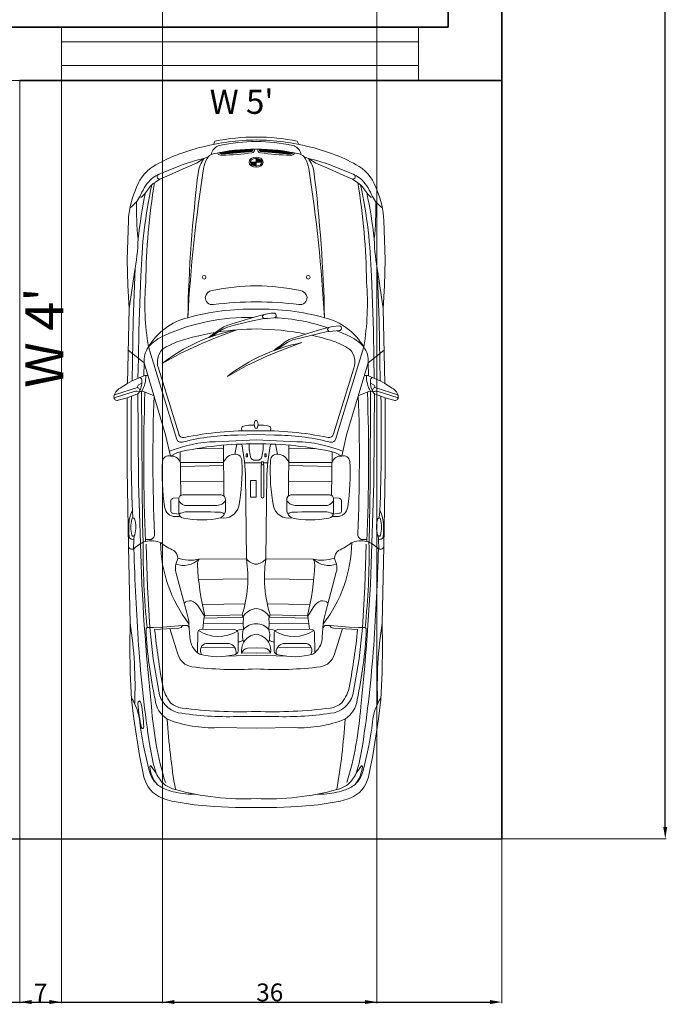
# Model space of a CAD drawing. Units: feet. Extents: x -297 to 770, y -228 to 625.
# Tile 4 of 14: x 661 to 770, y -228 to -62. Entities that reach past the tile are written whole.
import ezdxf

# ---------------------------------------------------------------- set-up
doc = ezdxf.new("R2010")
doc.units = ezdxf.units.FT
doc.header["$MEASUREMENT"] = 0
for name, color, linetype, lineweight in [('A-ANNO-DIMS', 2, 'Continuous', 18), ('A-ANNO-TEXT', 7, 'Continuous', 18), ('A-EQPM-VEHI', 8, 'Continuous', 13), ('A-EQPM-VEHI-PATT', 9, 'Continuous', 13), ('A-FLOR-EDGE', 7, 'Continuous', 25), ('A-WALL', 7, 'Continuous', 35), ('windows', 30, 'Continuous', 18)]:
    doc.layers.add(name, color=color, linetype=linetype, lineweight=lineweight)
doc.styles.add('Annotative', font='arial.ttf')
doc.styles.get("Standard").update_dxf_attribs({"font": 'arial.ttf'})
doc.dimstyles.get("Standard").update_dxf_attribs({"dimtxt": 3, "dimasz": 2, "dimexe": 0.18, "dimexo": 0.0625, "dimgap": 0.09, "dimtad": 1, "dimtoh": 1, "dimdec": 1, "dimzin": 0, "dimdsep": 46, "dimlunit": 3, "dimtxsty": 'Standard', "dimcen": 0, "dimclre": 256, "dimadec": 0, "dimazin": 0, "dimtfac": 1, "dimtdec": 1, "dimtofl": 0, "dimtmove": 0, "dimatfit": 3, "dimfxl": 1, "dimtolj": 1, "dimtzin": 0, "dimlwe": -1, "dimarcsym": 0})

# ---------------------------------------------------------------- blocks, each defined once
blk = doc.blocks.new('WIN-5FT')
for p, q in [((60, 6.5), (0, 6.5)), ((60, 2.5), (0, 2.5))]:
    blk.add_line(p, q)
blk.add_lwpolyline([(60, 0), (60, 9), (0, 9), (0, 0)], close=True)
blk = doc.blocks.new('*D43')
at = {"layer": 'A-ANNO-DIMS', "transparency": 16777216}
for p, q in [((382.16, -173.1), (382.16, -227.67)), ((742.16, -200.1), (742.16, -227.67))]:
    blk.add_line(p, q, dxfattribs=at)
at = {"layer": 'A-ANNO-DIMS', "color": 0, "lineweight": -2, "transparency": 16777216}
blk.add_line((384.16, -227.49), (740.16, -227.49), dxfattribs=at)
at = {"layer": 'A-ANNO-DIMS', "color": 0, "transparency": 16777216}
for points in [[(384.16, -227.15), (384.16, -227.82), (382.16, -227.49)], [(740.16, -227.15), (740.16, -227.82), (742.16, -227.49)]]:
    blk.add_solid(points, dxfattribs=at)
at = {"layer": 'Defpoints', "color": 0, "transparency": 16777216}
for p in [(382.16, -173.04), (742.16, -200.04), (742.16, -227.49)]:
    blk.add_point(p, dxfattribs=at)
at = {"layer": 'A-ANNO-DIMS', "color": 0, "transparency": 16777216, "insert": (562.16, -225.86), "char_height": 3, "attachment_point": 5}
blk.add_mtext('\\A1;360', dxfattribs=at)
blk = doc.blocks.new('*D44')
at = {"layer": 'A-ANNO-DIMS', "transparency": 16777216}
for p, q in [((742.22, 306.96), (769.79, 306.96)), ((742.22, -200.04), (769.79, -200.04))]:
    blk.add_line(p, q, dxfattribs=at)
at = {"layer": 'A-ANNO-DIMS', "color": 0, "lineweight": -2, "transparency": 16777216}
blk.add_line((769.61, -198.04), (769.61, 304.96), dxfattribs=at)
at = {"layer": 'A-ANNO-DIMS', "color": 0, "transparency": 16777216}
for points in [[(769.27, 304.96), (769.94, 304.96), (769.61, 306.96)], [(769.27, -198.04), (769.94, -198.04), (769.61, -200.04)]]:
    blk.add_solid(points, dxfattribs=at)
at = {"layer": 'Defpoints', "color": 0, "transparency": 16777216}
for p in [(742.16, 306.96), (769.61, 306.96), (742.16, -200.04)]:
    blk.add_point(p, dxfattribs=at)
at = {"layer": 'A-ANNO-DIMS', "color": 0, "transparency": 16777216, "insert": (767.98, 53.46), "char_height": 3, "attachment_point": 5, "rotation": 90}
blk.add_mtext('\\A1;507', dxfattribs=at)
blk = doc.blocks.new('*D56')
at = {"layer": 'A-ANNO-DIMS', "transparency": 16777216}
for p, q in [((742.09, -72.54), (354.53, -72.54)), ((742.09, -200.04), (354.53, -200.04))]:
    blk.add_line(p, q, dxfattribs=at)
at = {"layer": 'A-ANNO-DIMS', "color": 0, "lineweight": -2, "transparency": 16777216}
blk.add_line((354.71, -74.54), (354.71, -198.04), dxfattribs=at)
at = {"layer": 'A-ANNO-DIMS', "color": 0, "transparency": 16777216}
for points in [[(354.37, -74.54), (355.04, -74.54), (354.71, -72.54)], [(354.37, -198.04), (355.04, -198.04), (354.71, -200.04)]]:
    blk.add_solid(points, dxfattribs=at)
at = {"layer": 'Defpoints', "color": 0, "transparency": 16777216}
for p in [(742.16, -72.54), (354.71, -200.04), (742.16, -200.04)]:
    blk.add_point(p, dxfattribs=at)
at = {"layer": 'A-ANNO-DIMS', "color": 0, "transparency": 16777216, "insert": (353.08, -136.29), "char_height": 3, "attachment_point": 5, "rotation": 90}
blk.add_mtext('\\A1;127.5', dxfattribs=at)
blk = doc.blocks.new('*D58')
at = {"layer": 'A-ANNO-DIMS', "transparency": 16777216}
for p, q in [((661.16, -72.6), (661.16, -227.67)), ((668.16, -72.6), (668.16, -227.67))]:
    blk.add_line(p, q, dxfattribs=at)
at = {"layer": 'A-ANNO-DIMS', "color": 0, "lineweight": -2, "transparency": 16777216}
blk.add_line((663.16, -227.49), (666.16, -227.49), dxfattribs=at)
at = {"layer": 'A-ANNO-DIMS', "color": 0, "transparency": 16777216}
for points in [[(663.16, -227.15), (663.16, -227.82), (661.16, -227.49)], [(666.16, -227.15), (666.16, -227.82), (668.16, -227.49)]]:
    blk.add_solid(points, dxfattribs=at)
at = {"layer": 'Defpoints', "color": 0, "transparency": 16777216}
for p in [(661.16, -72.54), (668.16, -72.54), (668.16, -227.49)]:
    blk.add_point(p, dxfattribs=at)
at = {"layer": 'A-ANNO-DIMS', "color": 0, "transparency": 16777216, "insert": (664.66, -225.9), "char_height": 3, "attachment_point": 5}
blk.add_mtext('\\A1;7', dxfattribs=at)
blk = doc.blocks.new('*D68')
at = {"layer": 'A-ANNO-DIMS', "transparency": 16777216}
for p, q in [((685.16, 306.9), (685.16, -227.67)), ((721.16, 306.9), (721.16, -227.67))]:
    blk.add_line(p, q, dxfattribs=at)
at = {"layer": 'A-ANNO-DIMS', "color": 0, "lineweight": -2, "transparency": 16777216}
blk.add_line((687.16, -227.49), (719.16, -227.49), dxfattribs=at)
at = {"layer": 'A-ANNO-DIMS', "color": 0, "transparency": 16777216}
for points in [[(687.16, -227.15), (687.16, -227.82), (685.16, -227.49)], [(719.16, -227.15), (719.16, -227.82), (721.16, -227.49)]]:
    blk.add_solid(points, dxfattribs=at)
at = {"layer": 'Defpoints', "color": 0, "transparency": 16777216}
for p in [(685.16, 306.96), (721.16, 306.96), (721.16, -227.49)]:
    blk.add_point(p, dxfattribs=at)
at = {"layer": 'A-ANNO-DIMS', "color": 0, "transparency": 16777216, "insert": (703.16, -225.86), "char_height": 3, "attachment_point": 5}
blk.add_mtext('\\A1;36', dxfattribs=at)

msp = doc.modelspace()

# ---------------------------------------------------------------- hatches: boundary and pattern name
at = {"layer": 'A-EQPM-VEHI-PATT'}
h = msp.add_hatch(dxfattribs=at)
h.set_pattern_fill('ANSI31', color=256, scale=0.200946, angle=30.004, style=0)
h.set_pattern_definition([(75.004, (382.155307, -173.037275), (-0.0242628202, 0.0064993876), [])])
h.paths.add_polyline_path([(694.646, -84.653), (694.683, -84.701), (694.726, -84.744), (694.774, -84.781), (694.826, -84.813), (694.881, -84.837), (694.939, -84.854), (694.999, -84.864), (695.059, -84.866), (695.12, -84.861), (695.681, -84.839), (696.241, -84.812), (696.801, -84.778), (697.361, -84.738), (697.921, -84.691), (698.479, -84.639), (699.038, -84.58), (699.595, -84.514), (700.152, -84.443), (700.189, -84.437), (700.225, -84.425), (700.258, -84.407), (700.287, -84.382), (700.31, -84.353), (700.329, -84.32), (700.34, -84.284), (700.345, -84.247), (700.343, -84.209), (700.334, -84.173), (700.319, -84.139), (700.297, -84.108), (700.27, -84.081), (700.239, -84.06), (700.126, -84.063), (700.014, -84.066), (699.901, -84.069), (699.789, -84.073), (699.676, -84.077), (699.564, -84.082), (699.451, -84.086), (699.339, -84.092), (699.226, -84.097), (699.114, -84.103), (699.001, -84.11), (698.889, -84.116), (698.776, -84.124), (698.664, -84.131), (698.552, -84.139), (698.439, -84.147), (698.327, -84.156), (698.215, -84.165), (698.103, -84.174), (697.991, -84.184), (697.878, -84.194), (697.766, -84.205), (697.654, -84.216), (697.542, -84.227), (697.43, -84.239), (697.318, -84.251), (697.206, -84.263), (697.094, -84.276), (696.983, -84.289), (696.871, -84.303), (696.759, -84.317), (696.647, -84.331), (696.536, -84.346), (696.424, -84.361), (696.313, -84.376), (696.201, -84.392), (696.09, -84.408), (695.978, -84.425), (695.867, -84.442), (695.756, -84.459), (695.644, -84.477), (695.533, -84.495), (695.422, -84.513), (695.311, -84.532), (695.2, -84.551), (695.089, -84.571), (694.979, -84.591), (694.868, -84.611), (694.757, -84.632)])
h = msp.add_hatch(dxfattribs=at)
h.set_pattern_fill('ANSI31', color=256, scale=0.200942, angle=30.004, style=0)
h.set_pattern_definition([(75.004, (382.155307, -173.037275), (-0.0242623372, 0.0064992583), [])])
h.paths.add_polyline_path([(701.519, -84.06), (701.488, -84.081), (701.461, -84.108), (701.439, -84.139), (701.424, -84.173), (701.415, -84.209), (701.413, -84.247), (701.418, -84.284), (701.429, -84.32), (701.448, -84.353), (701.471, -84.382), (701.5, -84.407), (701.533, -84.425), (701.569, -84.437), (701.606, -84.443), (702.163, -84.514), (702.72, -84.58), (703.278, -84.639), (703.837, -84.691), (704.397, -84.738), (704.956, -84.778), (705.517, -84.812), (706.077, -84.839), (706.638, -84.861), (706.699, -84.866), (706.759, -84.864), (706.819, -84.854), (706.877, -84.837), (706.932, -84.813), (706.984, -84.781), (707.032, -84.744), (707.075, -84.701), (707.111, -84.653), (707.001, -84.632), (706.89, -84.611), (706.779, -84.591), (706.669, -84.571), (706.558, -84.551), (706.447, -84.532), (706.336, -84.513), (706.225, -84.495), (706.113, -84.477), (706.002, -84.459), (705.891, -84.442), (705.78, -84.425), (705.668, -84.408), (705.557, -84.392), (705.445, -84.376), (705.334, -84.361), (705.222, -84.346), (705.111, -84.331), (704.999, -84.317), (704.887, -84.303), (704.775, -84.289), (704.664, -84.276), (704.552, -84.263), (704.44, -84.251), (704.328, -84.239), (704.216, -84.227), (704.104, -84.216), (703.992, -84.205), (703.88, -84.194), (703.767, -84.184), (703.655, -84.174), (703.543, -84.165), (703.431, -84.156), (703.318, -84.147), (703.206, -84.139), (703.094, -84.131), (702.981, -84.124), (702.869, -84.116), (702.757, -84.11), (702.644, -84.103), (702.532, -84.097), (702.419, -84.092), (702.307, -84.086), (702.194, -84.082), (702.082, -84.077), (701.969, -84.073), (701.857, -84.069), (701.744, -84.066), (701.632, -84.063)])
h = msp.add_hatch(color=256, dxfattribs=at)
edge = h.paths.add_edge_path()
edge.add_line((700.879, -86.271), (700.879, -85.631))
edge.add_spline(control_points=[(700.879, -85.631), (701.04, -85.631), (701.2, -85.658), (701.678, -85.83), (701.857, -86.049), (701.857, -86.271)], knot_values=[6.2672483, 6.2672483, 6.2672483, 6.2672483, 6.732595, 6.732595, 7.8539816, 7.8539816, 7.8539816, 7.8539816], degree=3, periodic=0)
edge.add_line((701.857, -86.271), (700.879, -86.271))
h = msp.add_hatch(color=256, dxfattribs=at)
edge = h.paths.add_edge_path()
edge.add_line((700.879, -86.271), (700.879, -86.915))
edge.add_spline(control_points=[(700.879, -86.915), (700.553, -86.915), (700.236, -86.793), (699.955, -86.516), (699.902, -86.393), (699.901, -86.271)], knot_values=[4.712389, 4.712389, 4.712389, 4.712389, 5.655061, 5.655061, 6.2672483, 6.2672483, 6.2672483, 6.2672483], degree=3, periodic=0)
edge.add_line((699.901, -86.271), (700.879, -86.271))

# ---------------------------------------------------------------- linework, layer by layer
at = {"layer": 'A-EQPM-VEHI'}
for p, q in [((693.964, -82.748), (693.722, -83.283)), ((707.794, -82.748), (708.036, -83.283)), ((688.627, -86.65), (690.666, -85.978)), ((690.666, -85.978), (692.112, -85.668)), ((692.112, -85.668), (690.847, -86.443)), ((692.112, -85.668), (692.817, -85.365)), ((693.4, -84.666), (693.386, -84.944)), ((700.879, -85.631), (700.879, -86.915)), ((708.358, -84.666), (708.372, -84.944)), ((709.646, -85.668), (708.941, -85.365)), ((711.091, -85.978), (709.646, -85.668)), ((709.646, -85.668), (710.911, -86.443)), ((713.131, -86.65), (711.091, -85.978)), ((685.115, -88.07), (688.627, -86.65)), ((688.601, -87.399), (686.251, -88.432)), ((690.847, -86.443), (688.601, -87.399)), ((699.901, -86.271), (700.879, -86.271)), ((701.857, -86.271), (700.879, -86.271)), ((710.911, -86.443), (713.157, -87.399)), ((716.642, -88.07), (713.131, -86.65)), ((713.157, -87.399), (715.506, -88.432)), ((684.702, -89.129), (683.954, -89.646)), ((686.251, -88.432), (684.702, -89.129)), ((715.506, -88.432), (717.056, -89.129)), ((717.056, -89.129), (717.804, -89.646)), ((682.766, -90.73), (682.095, -91.634)), ((718.992, -90.73), (719.663, -91.634)), ((682.095, -91.634), (681.682, -92.074)), ((719.663, -91.634), (720.076, -92.074)), ((679.41, -96.044), (679.227, -102.695)), ((722.348, -96.044), (722.531, -102.695)), ((679.227, -102.695), (679.313, -106.998)), ((680.554, -104.049), (680.201, -112.961)), ((721.204, -104.049), (721.557, -112.961)), ((722.531, -102.695), (722.445, -106.998)), ((680.416, -104.781), (679.518, -110.872)), ((681.527, -105.38), (681.191, -114.601)), ((720.231, -105.38), (720.567, -114.601)), ((721.341, -104.781), (722.24, -110.872)), ((679.313, -106.998), (679.518, -110.872)), ((722.445, -106.998), (722.24, -110.872)), ((679.518, -110.872), (679.278, -123.501)), ((722.24, -110.872), (722.48, -123.501)), ((701.337, -112.092), (699.617, -112.581)), ((702.518, -111.823), (701.337, -112.092)), ((701.69, -112.654), (702.142, -112.562)), ((701.926, -112.216), (701.94, -112.101)), ((701.998, -112.408), (701.926, -112.216)), ((701.94, -112.101), (702.051, -111.963)), ((702.142, -112.562), (701.998, -112.408)), ((702.051, -111.963), (702.166, -111.903)), ((702.142, -112.562), (702.791, -112.543)), ((703.381, -111.678), (702.518, -111.823)), ((702.791, -112.543), (703.835, -112.436)), ((703.796, -111.654), (703.381, -111.678)), ((703.796, -111.654), (703.796, -111.654)), ((703.835, -112.436), (703.835, -112.436)), ((680.201, -112.961), (680.046, -123.059)), ((695.455, -113.938), (694.814, -114.343)), ((695.265, -114.368), (696.073, -113.996)), ((695.973, -113.737), (695.455, -113.938)), ((699.617, -112.581), (695.973, -113.737)), ((696.073, -113.996), (697.228, -113.689)), ((697.228, -113.689), (700.282, -112.955)), ((700.282, -112.955), (701.69, -112.654)), ((713.481, -113.979), (712.3, -114.248)), ((712.903, -114.257), (713.014, -114.119)), ((713.014, -114.119), (713.129, -114.059)), ((714.344, -113.834), (713.481, -113.979)), ((714.759, -113.81), (714.344, -113.834)), ((714.759, -113.81), (714.759, -113.81)), ((721.557, -112.961), (721.712, -123.059)), ((681.191, -114.601), (681.09, -119.232)), ((691.732, -116.744), (694.354, -115.672)), ((693.249, -115.488), (692.949, -115.758)), ((694.092, -114.854), (693.249, -115.488)), ((693.411, -115.59), (694.295, -114.964)), ((694.814, -114.343), (694.092, -114.854)), ((694.295, -114.964), (695.265, -114.368)), ((694.354, -115.672), (697.617, -114.453)), ((710.58, -114.736), (706.936, -115.893)), ((707.036, -116.152), (708.191, -115.845)), ((708.191, -115.845), (711.245, -115.11)), ((712.3, -114.248), (710.58, -114.736)), ((711.245, -115.11), (712.653, -114.81)), ((712.653, -114.81), (713.105, -114.718)), ((712.889, -114.372), (712.903, -114.257)), ((712.961, -114.564), (712.889, -114.372)), ((713.105, -114.718), (712.961, -114.564)), ((713.105, -114.718), (713.754, -114.699)), ((713.754, -114.699), (714.798, -114.592)), ((714.798, -114.592), (714.798, -114.592)), ((720.567, -114.601), (720.668, -119.232)), ((682.792, -117.339), (687.544, -132.898)), ((688.215, -118.368), (691.732, -116.744)), ((705.055, -117.01), (704.212, -117.644)), ((704.374, -117.746), (705.258, -117.12)), ((705.777, -116.499), (705.055, -117.01)), ((705.258, -117.12), (706.228, -116.524)), ((705.317, -117.828), (708.58, -116.609)), ((706.418, -116.093), (705.777, -116.499)), ((706.228, -116.524), (707.036, -116.152)), ((706.936, -115.893), (706.418, -116.093)), ((718.966, -117.339), (714.214, -132.898)), ((679.385, -117.896), (682.085, -120.012)), ((685.087, -120.129), (688.215, -118.368)), ((699.178, -120.524), (702.695, -118.9)), ((702.695, -118.9), (705.317, -117.828)), ((704.212, -117.644), (703.912, -117.914)), ((722.373, -117.896), (719.673, -120.012)), ((681.09, -119.232), (681.028, -122.633)), ((682.085, -120.012), (682.008, -122.207)), ((682.085, -120.012), (685.674, -132.099)), ((696.05, -122.285), (699.178, -120.524)), ((719.673, -120.012), (716.084, -132.099)), ((719.673, -120.012), (719.75, -122.207)), ((720.668, -119.232), (720.73, -122.633)), ((682.008, -122.207), (680.046, -123.059)), ((684.446, -120.889), (687.88, -131.917)), ((717.312, -120.889), (713.878, -131.917)), ((719.75, -122.207), (721.712, -123.059)), ((680.921, -124.168), (677.075, -125.393)), ((679.278, -123.501), (678.008, -124.278)), ((680.046, -123.059), (679.278, -123.501)), ((681.675, -123.437), (681.069, -123.783)), ((720.083, -123.437), (720.689, -123.783)), ((720.837, -124.168), (724.683, -125.393)), ((721.712, -123.059), (722.48, -123.501)), ((722.48, -123.501), (723.75, -124.278)), ((680.363, -124.8), (677.008, -125.91)), ((680.827, -125.275), (679.191, -125.879)), ((681.015, -125.181), (681.055, -131.504)), ((681.643, -124.752), (681.703, -140.477)), ((683.722, -125.526), (681.958, -124.821)), ((718.036, -125.526), (719.8, -124.821)), ((720.115, -124.752), (720.055, -140.477)), ((720.743, -125.181), (720.703, -131.504)), ((720.931, -125.275), (722.567, -125.879)), ((721.395, -124.8), (724.75, -125.91)), ((679.191, -125.879), (677.724, -126.293)), ((679.191, -125.879), (679.208, -137.861)), ((722.567, -125.879), (722.55, -137.861)), ((722.567, -125.879), (724.034, -126.293)), ((700.722, -129.728), (700.985, -129.728)), ((681.055, -131.504), (681.136, -140.234)), ((685.674, -132.099), (686.5, -135.689)), ((697.788, -132.186), (700.879, -132.078)), ((698.44, -131.022), (698.447, -131.436)), ((700.714, -130.985), (701.022, -130.985)), ((703.97, -132.186), (700.879, -132.078)), ((703.318, -131.022), (703.311, -131.436)), ((716.084, -132.099), (715.258, -135.689)), ((720.703, -131.504), (720.622, -140.234)), ((694.063, -133.266), (700.879, -132.969)), ((695.399, -133.836), (695.427, -142.379)), ((697.651, -133.684), (697.275, -135.367)), ((698.935, -136.618), (698.468, -133.651)), ((707.695, -133.266), (700.879, -132.969)), ((702.823, -136.618), (703.29, -133.651)), ((704.107, -133.684), (704.483, -135.367)), ((706.359, -133.836), (706.331, -142.379)), ((687.681, -135.063), (686.5, -135.689)), ((688.106, -134.967), (688.22, -142.305)), ((691.044, -134.392), (695.401, -134.474)), ((699.194, -135.327), (699.194, -135.805)), ((699.402, -135.327), (699.194, -135.327)), ((699.402, -135.805), (699.402, -135.327)), ((702.356, -135.805), (702.356, -135.327)), ((702.356, -135.327), (702.563, -135.327)), ((702.563, -135.327), (702.563, -135.805)), ((710.714, -134.392), (706.357, -134.474)), ((713.652, -134.967), (713.538, -142.305)), ((714.077, -135.063), (715.258, -135.689)), ((688.134, -136.78), (695.409, -136.739)), ((688.145, -137.446), (695.41, -137.258)), ((699.093, -138.795), (698.935, -136.618)), ((698.95, -136.82), (700.879, -136.82)), ((699.194, -135.805), (699.402, -135.805)), ((700.617, -136.38), (700.879, -136.379)), ((701.141, -136.38), (700.879, -136.379)), ((701.799, -136.82), (700.879, -136.82)), ((702.178, -137.168), (701.696, -137.168)), ((701.696, -137.168), (701.696, -142.5)), ((701.799, -137.168), (701.799, -136.628)), ((701.799, -136.628), (702.093, -136.628)), ((702.093, -137.168), (701.799, -137.168)), ((702.093, -136.628), (702.093, -137.168)), ((702.808, -136.82), (702.093, -136.82)), ((702.178, -142.5), (702.178, -137.168)), ((702.563, -135.805), (702.356, -135.805)), ((702.665, -138.795), (702.823, -136.618)), ((713.613, -137.446), (706.348, -137.258)), ((713.624, -136.78), (706.349, -136.739)), ((679.208, -137.861), (679.414, -150.924)), ((699.251, -152.988), (699.093, -138.795)), ((702.507, -152.988), (702.665, -138.795)), ((722.55, -137.861), (722.344, -150.924)), ((681.136, -140.234), (681.298, -145.207)), ((681.703, -140.477), (681.811, -147.099)), ((688.184, -140.022), (695.419, -139.938)), ((699.923, -139.792), (699.923, -142.591)), ((700.873, -139.792), (699.923, -139.792)), ((700.873, -142.591), (700.873, -139.792)), ((713.574, -140.022), (706.339, -139.938)), ((720.055, -140.477), (719.947, -147.099)), ((720.622, -140.234), (720.46, -145.207)), ((688.551, -142.224), (695.011, -142.224)), ((713.207, -142.224), (706.747, -142.224)), ((686.53, -143.094), (686.54, -145.002)), ((687.927, -142.683), (686.927, -142.781)), ((687.907, -142.889), (687.907, -145.258)), ((689.32, -143.99), (694.056, -143.97)), ((695.738, -143.055), (695.738, -144.946)), ((699.923, -142.591), (700.873, -142.591)), ((706.02, -143.055), (706.02, -144.946)), ((712.438, -143.99), (707.702, -143.97)), ((713.831, -142.683), (714.831, -142.781)), ((713.851, -142.889), (713.851, -145.258)), ((715.228, -143.094), (715.218, -145.002)), ((680.082, -144.883), (680.185, -146.086)), ((681.298, -145.207), (681.437, -150.403)), ((687.916, -145.443), (686.906, -145.294)), ((713.842, -145.443), (714.852, -145.294)), ((720.46, -145.207), (720.321, -150.403)), ((721.676, -144.883), (721.573, -146.086)), ((681.811, -147.099), (681.92, -150.165)), ((687.346, -145.84), (688.115, -145.861)), ((714.412, -145.84), (713.643, -145.861)), ((719.947, -147.099), (719.838, -150.165)), ((679.484, -147.373), (679.502, -148.752)), ((679.502, -148.752), (679.556, -149.29)), ((722.256, -148.752), (722.202, -149.29)), ((722.274, -147.373), (722.256, -148.752)), ((680.335, -149.693), (680.013, -149.675)), ((680.335, -149.693), (680.29, -151.305)), ((680.335, -149.693), (680.38, -149.12)), ((682.279, -149.699), (683.216, -149.693)), ((682.391, -150.47), (682.608, -157.733)), ((719.479, -149.699), (718.542, -149.693)), ((719.367, -150.47), (719.149, -157.733)), ((721.423, -149.693), (721.378, -149.12)), ((721.423, -149.693), (721.745, -149.675)), ((721.423, -149.693), (721.468, -151.305)), ((679.414, -150.924), (679.721, -163.793)), ((722.344, -150.924), (722.037, -163.793)), ((687.711, -152.901), (687.38, -153.841)), ((691.279, -153.002), (699.251, -152.988)), ((710.479, -153.002), (702.507, -152.988)), ((714.047, -152.901), (714.378, -153.841)), ((687.411, -155.214), (689.215, -162.033)), ((714.347, -155.214), (712.542, -162.033)), ((691.2, -156.449), (699.487, -156.315)), ((710.558, -156.449), (702.271, -156.315)), ((682.608, -157.733), (683.008, -164.524)), ((719.149, -157.733), (718.75, -164.524)), ((691.838, -160.624), (699.016, -160.513)), ((709.92, -160.624), (702.742, -160.513)), ((691.212, -160.991), (692.197, -162.613)), ((710.546, -160.991), (709.561, -162.613)), ((679.721, -163.793), (679.67, -167.667)), ((689.594, -163.898), (689.762, -166.153)), ((692.115, -163.001), (691.919, -164.81)), ((692.019, -163.882), (698.698, -163.786)), ((692.197, -162.613), (692.115, -163.001)), ((692.126, -162.949), (698.624, -162.794)), ((692.197, -162.613), (692.276, -162.524)), ((692.276, -162.524), (698.514, -162.395)), ((698.514, -162.395), (698.624, -162.794)), ((698.624, -162.794), (698.752, -162.94)), ((698.752, -162.94), (698.698, -163.786)), ((698.698, -163.786), (698.734, -164.864)), ((703.134, -162.794), (703.006, -162.94)), ((703.006, -162.94), (703.06, -163.786)), ((703.06, -163.786), (703.024, -164.864)), ((709.739, -163.882), (703.06, -163.786)), ((703.244, -162.395), (703.134, -162.794)), ((709.632, -162.949), (703.134, -162.794)), ((709.482, -162.524), (703.244, -162.395)), ((709.561, -162.613), (709.482, -162.524)), ((709.561, -162.613), (709.643, -163.001)), ((709.643, -163.001), (709.839, -164.81)), ((712.164, -163.898), (711.996, -166.153)), ((722.037, -163.793), (722.088, -167.667)), ((683.61, -164.522), (682.572, -164.524)), ((683.008, -164.524), (683.589, -169.753)), ((685.208, -164.444), (683.61, -164.522)), ((687.907, -164.615), (683.828, -164.847)), ((688.481, -164.196), (685.208, -164.444)), ((686.351, -164.703), (687.737, -169.006)), ((688.481, -164.196), (689.312, -164.197)), ((691.096, -165.314), (691.021, -168.738)), ((691.919, -164.81), (691.498, -164.883)), ((691.919, -164.81), (697.265, -164.864)), ((697.61, -164.991), (698, -164.876)), ((698, -164.876), (698.734, -164.864)), ((703.758, -164.876), (703.024, -164.864)), ((704.148, -164.991), (703.758, -164.876)), ((709.839, -164.81), (704.493, -164.864)), ((709.839, -164.81), (710.26, -164.883)), ((710.662, -165.314), (710.737, -168.738)), ((713.277, -164.196), (712.446, -164.197)), ((713.277, -164.196), (716.55, -164.444)), ((713.851, -164.615), (717.93, -164.847)), ((715.407, -164.703), (714.021, -169.006)), ((716.55, -164.444), (718.148, -164.522)), ((718.148, -164.522), (719.186, -164.524)), ((718.75, -164.524), (718.169, -169.753)), ((697.865, -168.476), (697.841, -165.635)), ((703.893, -168.476), (703.917, -165.635)), ((679.67, -167.667), (679.721, -172.039)), ((691.622, -167.852), (697.253, -167.79)), ((692.504, -167.215), (696.347, -167.215)), ((698.444, -168.841), (700.879, -168.779)), ((700.879, -167.925), (699.439, -167.969)), ((700.879, -167.925), (702.319, -167.969)), ((703.314, -168.841), (700.879, -168.779)), ((710.136, -167.852), (704.505, -167.79)), ((709.254, -167.215), (705.411, -167.215)), ((722.088, -167.667), (722.037, -172.039)), ((683.589, -169.753), (684.533, -175.2)), ((695.838, -169.335), (700.879, -169.174)), ((705.92, -169.335), (700.879, -169.174)), ((718.169, -169.753), (717.225, -175.2)), ((679.721, -172.039), (679.946, -176.597)), ((722.037, -172.039), (721.812, -176.597)), ((679.946, -176.597), (680.34, -179.871)), ((721.812, -176.597), (721.418, -179.871)), ((680.34, -179.871), (681.3, -186.025)), ((697.701, -179.48), (700.879, -179.48)), ((704.057, -179.48), (700.879, -179.48)), ((721.418, -179.871), (720.458, -186.025)), ((694.429, -181.332), (700.879, -181.456)), ((707.329, -181.332), (700.879, -181.456)), ((681.3, -186.025), (681.917, -189.077)), ((720.458, -186.025), (719.841, -189.077)), ((684.08, -189.003), (683.227, -187.819)), ((717.678, -189.003), (718.531, -187.819)), ((689.44, -192.515), (690.582, -192.521)), ((712.318, -192.515), (711.176, -192.521)), ((687.458, -193.828), (690.457, -194.308)), ((690.457, -194.308), (693.884, -194.6)), ((693.884, -194.6), (697.425, -194.755)), ((697.425, -194.755), (700.879, -194.772)), ((704.333, -194.755), (700.879, -194.772)), ((707.873, -194.6), (704.333, -194.755)), ((711.301, -194.308), (707.873, -194.6)), ((714.3, -193.828), (711.301, -194.308))]:
    msp.add_line(p, q, dxfattribs=at)
for centre in [(692.139, -105.615), (709.619, -105.615)]:
    msp.add_circle(centre, 0.307, dxfattribs=at)
for centre, radius, start, end in [((701.495, -122.515), 39.995, 90.88313, 104.19911), ((700.685, -114.501), 32.457, 89.65731, 101.95036), ((700.879, -110.093), 27.318, 89.99964, 102.97383), ((701.073, -114.501), 32.457, 78.04964, 90.34269), ((700.263, -122.515), 39.995, 75.80089, 89.11687), ((700.879, -110.093), 27.318, 77.02617, 90.00036), ((699.101, -114.202), 31.349, 103.68324, 119.69352), ((695.114, -85.244), 1.808, 101.74541, 161.36532), ((700.952, -117.482), 33.429, 90.12545, 102.57191), ((700.142, -84.239), 0.204, 272.78275, 61.54503), ((700.142, -84.239), 0.45, 274.38011, 24.12714), ((700.806, -117.482), 33.429, 77.42809, 89.87455), ((701.616, -84.239), 0.45, 155.87286, 265.61989), ((701.616, -84.239), 0.204, 118.45497, 267.21725), ((706.644, -85.244), 1.808, 18.63468, 78.25459), ((702.657, -114.202), 31.349, 60.30648, 76.31676), ((696.339, -88.795), 5.258, 143.50289, 168.70969), ((696.822, -88.055), 4.834, 150.23963, 171.47764), ((693.974, -86.333), 1.509, 101.38802, 153.30988), ((695.046, -84.385), 0.729, 205.91225, 277.4566), ((695.046, -84.385), 0.482, 213.85525, 278.74787), ((693.522, -35.133), 49.753, 271.84014, 277.65755), ((693.522, -35.133), 50, 271.85547, 277.64785), ((708.236, -35.133), 50, 262.35215, 268.14453), ((708.236, -35.133), 49.753, 262.34245, 268.15986), ((706.712, -84.385), 0.729, 262.5434, 334.08775), ((706.712, -84.385), 0.482, 261.25213, 326.14475), ((707.784, -86.333), 1.509, 26.69012, 78.61198), ((704.936, -88.055), 4.834, 8.52236, 29.76037), ((705.419, -88.795), 5.258, 11.29031, 36.49711), ((687.697, -93.15), 7.431, 123.71939, 163.72515), ((943.023, -126.461), 254.012, 171.14022, 176.82946), ((458.735, -126.461), 254.012, 3.17054, 8.85978), ((714.061, -93.15), 7.431, 16.27485, 56.28061), ((691.336, -96.394), 10.919, 139.36893, 156.54162), ((687.204, -93.988), 6.275, 109.43758, 131.44791), ((684.642, -88.71), 0.411, 109.44152, 285.61385), ((923.595, -116.972), 234.24, 172.83741, 178.88446), ((478.163, -116.972), 234.24, 1.11554, 7.16259), ((714.554, -93.988), 6.275, 48.55209, 70.56242), ((717.116, -88.71), 0.411, 254.38615, 70.55848), ((710.422, -96.394), 10.919, 23.45838, 40.63107), ((763.658, -107.317), 82.154, 167.87467, 178.64951), ((793.974, -107.905), 111.656, 170.62903, 179.23454), ((685.291, -92.303), 2.975, 116.72328, 148.09101), ((716.467, -92.303), 2.975, 31.90899, 63.27672), ((607.784, -107.905), 111.656, 0.76546, 9.37097), ((638.1, -107.317), 82.154, 1.35049, 12.12533), ((694.007, -96.804), 14.617, 156.89133, 177.01886), ((676.489, -89.525), 5.45, 305.73696, 332.43387), ((768.484, -109.185), 88.019, 168.32761, 173.47041), ((681.524, -91.983), 0.182, 184.22212, 330.13213), ((633.274, -109.185), 88.019, 6.52959, 11.67239), ((720.234, -91.983), 0.182, 209.86787, 355.77788), ((725.269, -89.525), 5.45, 207.56613, 234.26304), ((707.751, -96.804), 14.617, 2.98114, 23.10867), ((728.407, -94.111), 47.641, 178.52289, 186.10313), ((673.351, -94.111), 47.641, 353.89687, 1.47711), ((648.851, -98.454), 32.193, 348.66672, 358.71512), ((752.907, -98.454), 32.193, 181.28488, 191.33328), ((726.995, -109.986), 44.811, 175.42757, 189.44408), ((701.323, -144.293), 37.265, 90.68282, 102.15134), ((700.435, -144.293), 37.265, 77.84866, 89.31718), ((674.763, -109.986), 44.811, 350.55592, 4.57243), ((693.508, -109.046), 1.179, 175.53481, 279.81226), ((693.638, -109.178), 1.325, 96.91169, 170.30328), ((708.25, -109.046), 1.179, 260.18773, 4.46519), ((708.12, -109.178), 1.325, 9.69672, 83.08831), ((702.166, -181.93), 72.219, 91.02136, 96.72537), ((699.592, -181.93), 72.219, 83.27463, 88.97864), ((691.926, -122.696), 10.59, 103.80565, 149.60976), ((699.596, -146.705), 34.341, 88.74333, 114.31335), ((700.165, -151.629), 40.668, 88.9934, 105.34945), ((701.593, -151.629), 40.668, 74.65055, 91.0066), ((703.873, -112.043), 0.396, 264.37062, 101.27333), ((702.162, -146.705), 34.341, 71.69981, 86.91458), ((709.832, -122.696), 10.59, 30.39024, 76.19435), ((714.837, -114.198), 0.396, 264.37062, 101.27333), ((688.384, -122.261), 7.45, 113.13226, 138.64342), ((703.212, -143.472), 29.554, 100.91311, 127.82774), ((701.307, -159.12), 44.819, 99.33267, 107.36365), ((701.307, -159.12), 44.819, 90.54721, 98.68541), ((700.451, -159.12), 44.819, 78.71375, 89.45279), ((700.451, -159.12), 44.819, 72.63635, 77.47065), ((702.162, -146.705), 34.341, 65.68665, 69.0705), ((713.374, -122.261), 7.45, 41.35658, 66.86774), ((685.915, -119.594), 3.853, 144.164, 186.22235), ((692.082, -128.255), 12.615, 109.21073, 123.51355), ((714.175, -145.628), 29.554, 100.91311, 127.82774), ((709.676, -128.255), 12.615, 56.48645, 70.78927), ((715.843, -119.594), 3.853, 353.77765, 35.836), ((687.386, -119.868), 3.113, 136.80673, 199.14003), ((714.372, -119.868), 3.113, 340.85997, 43.19327), ((681.154, -122.963), 0.532, 352.61924, 65.14151), ((677.766, -122.358), 4.572, 328.44435, 2.80143), ((682.38, -123.114), 0.98, 68.72379, 112.2852), ((719.378, -123.114), 0.98, 67.7148, 111.27621), ((723.992, -122.358), 4.572, 177.19857, 211.55565), ((720.604, -122.963), 0.532, 114.85849, 187.38076), ((681.358, -124.115), 0.44, 130.97083, 186.96723), ((680.834, -124.651), 0.491, 324.13309, 79.83562), ((678.013, -123.174), 3.671, 331.26149, 2.21652), ((723.745, -123.174), 3.671, 177.78348, 208.73851), ((720.924, -124.651), 0.491, 100.16438, 215.86691), ((720.4, -124.115), 0.44, 353.03277, 49.02917), ((678.954, -126.017), 1.979, 118.55159, 172.40816), ((677.539, -125.777), 0.548, 177.69248, 289.69672), ((1028.97, -132.339), 349.113, 178.89534, 182.05902), ((680.621, -125.976), 1.204, 59.51211, 102.38611), ((680.603, -124.592), 0.719, 288.20227, 331.15262), ((681.674, -125.364), 0.613, 62.40843, 136.09685), ((997.908, -136.209), 315.917, 177.95117, 182.50706), ((974.758, -136.016), 291.225, 177.9357, 182.50028), ((427, -136.016), 291.225, 357.49972, 2.0643), ((403.85, -136.209), 315.917, 357.49294, 2.04883), ((720.084, -125.364), 0.613, 43.90315, 117.59157), ((721.137, -125.976), 1.204, 77.61389, 120.48789), ((721.155, -124.592), 0.719, 208.84738, 251.79773), ((372.788, -132.339), 349.113, 357.94098, 1.10466), ((722.804, -126.017), 1.979, 7.59184, 61.44841), ((724.219, -125.777), 0.548, 250.30328, 2.30752), ((698.817, -131.003), 0.377, 103.54974, 182.76386), ((700.2, -137.27), 6.794, 86.88903, 102.51243), ((701.903, -130.364), 1.342, 151.7301, 207.58465), ((700.083, -130.384), 1.115, 327.38983, 36.03523), ((701.558, -137.27), 6.794, 77.48757, 93.11097), ((702.941, -131.003), 0.377, 357.23614, 76.45026), ((688.632, -131.825), 0.758, 186.99823, 282.79745), ((697.427, -167.145), 34.961, 89.40858, 104.46932), ((699.812, -184.955), 53.536, 88.85755, 101.86962), ((701.946, -184.955), 53.536, 78.13038, 91.14245), ((704.33, -167.145), 34.961, 75.53068, 90.59142), ((713.126, -131.825), 0.758, 257.20255, 353.00177), ((694.578, -155.087), 21.827, 91.35001, 112.24403), ((688.202, -132.669), 0.697, 199.20691, 276.63373), ((700.277, -189.37), 55.748, 89.38179, 103.05861), ((652.745, 80.416), 216.711, 279.43817, 279.54793), ((706.137, -133.953), 6.456, 177.08701, 199.2679), ((701.48, -189.37), 55.748, 76.94139, 90.61821), ((695.621, -133.953), 6.456, 340.7321, 2.91299), ((707.18, -155.087), 21.827, 67.75597, 88.64999), ((749.012, 80.416), 216.711, 260.45207, 260.56183), ((713.556, -132.669), 0.697, 263.36627, 340.79309), ((686.191, -136.692), 1.05, 72.87734, 175.70582), ((686.667, -137.208), 1.528, 16.26696, 96.27372), ((697.358, -137.435), 2.07, 92.27741, 160.33698), ((697.367, -136.486), 1.123, 352.40221, 94.69008), ((704.391, -136.486), 1.123, 85.30992, 187.59779), ((704.4, -137.435), 2.07, 19.66302, 87.72259), ((715.091, -137.208), 1.528, 83.72628, 163.73304), ((715.567, -136.692), 1.05, 4.29418, 107.12266), ((721.981, -138.729), 36.898, 176.71333, 188.58914), ((667.266, -138.21), 31.254, 349.14696, 2.88868), ((700.719, -135.479), 0.907, 221.78401, 263.50019), ((701.039, -135.479), 0.907, 276.49981, 318.21599), ((734.492, -138.21), 31.254, 177.11132, 190.85304), ((679.776, -138.729), 36.898, 351.41086, 3.28667), ((688.527, -142.845), 0.622, 87.78964, 184.04866), ((694.957, -143.005), 0.783, 356.32352, 86.02894), ((706.801, -143.005), 0.783, 93.97106, 183.67648), ((713.231, -142.845), 0.622, 355.95134, 92.21036), ((687.145, -143.468), 0.72, 107.65434, 148.74648), ((689.18, -142.579), 1.418, 206.21187, 275.66112), ((694.231, -142.11), 1.868, 264.60231, 323.78273), ((701.937, -142.5), 0.241, 180, 0), ((707.527, -142.11), 1.868, 216.21727, 275.39769), ((712.578, -142.579), 1.418, 264.33888, 333.78813), ((714.613, -143.468), 0.72, 31.25352, 72.34566), ((684.987, -147.377), 5.503, 153.04375, 179.955), ((687.279, -144.049), 1.792, 186.10928, 272.14083), ((686.879, -144.952), 0.343, 188.42849, 274.4357), ((688.728, -145.312), 0.823, 176.22994, 264.4882), ((689.296, -147.731), 2.672, 96.4485, 121.10596), ((690.974, -237.989), 92.935, 87.75311, 91.21977), ((694.743, -146.359), 1.24, 48.47018, 95.76384), ((695.417, -143.508), 2.611, 258.74141, 347.02218), ((694.181, -144.662), 1.583, 297.30865, 349.65226), ((706.341, -143.508), 2.611, 192.97782, 281.25859), ((707.577, -144.662), 1.583, 190.34774, 242.69135), ((707.015, -146.359), 1.24, 84.23616, 131.52982), ((710.783, -237.989), 92.935, 88.78023, 92.24689), ((712.462, -147.731), 2.672, 58.89404, 83.5515), ((713.03, -145.312), 0.823, 275.5118, 3.77006), ((714.479, -144.049), 1.792, 267.85917, 353.89072), ((714.879, -144.952), 0.343, 265.5643, 351.57151), ((716.771, -147.377), 5.503, 0.045, 26.95625), ((685.664, -147.595), 5.831, 166.87128, 193.88233), ((680.227, -146.331), 0.248, 24.9407, 166.0475), ((675.765, -147.634), 4.894, 344.40912, 16.72129), ((691.624, -130.724), 15.692, 259.07032, 282.07714), ((710.134, -130.724), 15.692, 257.92286, 280.92968), ((725.993, -147.634), 4.894, 163.27871, 195.59088), ((721.531, -146.331), 0.248, 13.9525, 155.0593), ((716.094, -147.595), 5.831, 346.11767, 13.12872), ((680.237, -148.924), 0.243, 196.81003, 353.97207), ((682.783, -148.761), 1.029, 294.92435, 2.23387), ((718.975, -148.761), 1.029, 177.76613, 245.07565), ((721.521, -148.924), 0.243, 186.02793, 343.18997), ((680.04, -149.18), 0.496, 192.83184, 266.87806), ((683.66, -154.319), 4.504, 107.66601, 137.66648), ((1022.794, -140.992), 341.487, 181.57908, 186.19023), ((798.253, -152.077), 116.348, 179.05839, 186.14099), ((683.195, -154.309), 4.375, 66.89972, 101.88537), ((707.869, -149.827), 23.064, 181.03213, 217.5934), ((691.476, -141.741), 10.775, 232.46126, 245.72461), ((693.889, -149.827), 23.064, 322.4066, 358.96787), ((710.282, -141.741), 10.775, 294.27539, 307.53874), ((718.563, -154.309), 4.375, 78.11463, 113.10028), ((378.963, -140.992), 341.487, 353.80977, 358.42092), ((603.505, -152.077), 116.348, 353.85901, 0.94161), ((718.098, -154.319), 4.504, 42.33352, 72.33399), ((721.718, -149.18), 0.496, 273.12194, 347.16816), ((680.042, -150.724), 0.632, 183.78112, 297.23725), ((1073.954, -139.893), 393.788, 181.65788, 184.02202), ((686.105, -152.865), 1.607, 358.7494, 54.13918), ((715.653, -152.865), 1.607, 125.86082, 181.2506), ((327.804, -139.893), 393.788, 355.97798, 358.34212), ((721.716, -150.724), 0.632, 242.76275, 356.21888), ((690.288, -154.464), 2.974, 167.91534, 194.61118), ((688.665, -150.33), 3.739, 249.91158, 314.37084), ((689.757, -147.144), 6.053, 250.2522, 284.56882), ((693.27, -154.058), 2.253, 152.06298, 176.05653), ((732.277, -152.303), 41.287, 182.22093, 194.33292), ((678.742, -156.113), 20.746, 342.37403, 8.66528), ((701.148, -151.434), 2.452, 219.32295, 263.69156), ((700.61, -151.434), 2.452, 276.30844, 320.67705), ((723.016, -156.113), 20.746, 171.33472, 197.62597), ((669.481, -152.303), 41.287, 345.66708, 357.77907), ((712.001, -147.144), 6.053, 255.43118, 289.7478), ((713.093, -150.33), 3.739, 225.62916, 290.08842), ((708.488, -154.058), 2.253, 3.94347, 27.93702), ((711.47, -154.464), 2.974, 345.38882, 12.08466), ((689.75, -161.323), 1.318, 78.16915, 136.82185), ((688.982, -162.545), 2.718, 34.8897, 67.54753), ((712.776, -162.545), 2.718, 112.45247, 145.1103), ((712.008, -161.323), 1.318, 43.17815, 101.83085), ((683.247, -164.214), 6.355, 2.8556, 20.07589), ((701.256, -164.303), 3.034, 97.14474, 150.17286), ((700.502, -164.303), 3.034, 29.82714, 82.85526), ((718.511, -164.214), 6.355, 159.92411, 177.1444), ((610.496, -174.408), 70.034, 357.63018, 8.71793), ((700.86, -166.65), 2.776, 89.60788, 139.96006), ((700.898, -166.65), 2.776, 40.03994, 90.39212), ((791.262, -174.408), 70.034, 171.28207, 182.36982), ((682.759, -164.853), 0.378, 119.56971, 188.65001), ((752.138, -161.815), 69.821, 182.53997, 192.24649), ((819.749, -150.337), 136.693, 186.09357, 190.10868), ((687.864, -163.952), 0.664, 273.76718, 338.48996), ((689.066, -164.737), 0.593, 10.75744, 65.43194), ((691.51, -165.297), 0.414, 91.70701, 182.37416), ((694.553, -160.043), 5.993, 236.05838, 302.08534), ((697.23, -165.491), 0.628, 346.70376, 86.72578), ((701.97, -165.829), 3.377, 163.39145, 199.5007), ((699.788, -165.829), 3.377, 340.4993, 16.60855), ((704.528, -165.491), 0.628, 93.27422, 193.29624), ((707.205, -160.043), 5.993, 237.91466, 303.94162), ((710.248, -165.297), 0.414, 357.62584, 88.29299), ((712.692, -164.737), 0.593, 114.56806, 169.24256), ((713.894, -163.952), 0.664, 201.51004, 266.23282), ((582.009, -150.337), 136.693, 349.89132, 353.90643), ((649.62, -161.815), 69.821, 347.75351, 357.46003), ((718.999, -164.853), 0.378, 351.34999, 60.43029), ((693.192, -166.082), 3.43, 181.17443, 238.02849), ((697.947, -165.785), 1.131, 265.19291, 311.17334), ((701.326, -168.392), 2.917, 150.50216, 188.84788), ((701.147, -168.395), 2.764, 95.57396, 148.63162), ((700.61, -168.395), 2.764, 31.36838, 84.42604), ((700.432, -168.392), 2.917, 351.15212, 29.49784), ((703.811, -165.785), 1.131, 228.82666, 274.80709), ((708.566, -166.082), 3.43, 301.97151, 358.82557), ((883.586, -153.479), 202.936, 183.96575, 188.76024), ((692.724, -168.385), 1.224, 154.16031, 214.76283), ((692.579, -168.248), 1.036, 94.18707, 157.50673), ((696.113, -168.585), 1.39, 34.85864, 80.28163), ((697.091, -168.299), 0.794, 276.4073, 347.13267), ((696.039, -168.623), 1.472, 345.08441, 34.42651), ((699.645, -169.208), 1.256, 99.45306, 163.00981), ((702.113, -169.208), 1.256, 16.99019, 80.54694), ((704.667, -168.299), 0.794, 192.86733, 263.5927), ((705.719, -168.623), 1.472, 145.57349, 194.91559), ((705.645, -168.585), 1.39, 99.71837, 145.14136), ((709.179, -168.248), 1.036, 22.49327, 85.81293), ((709.034, -168.385), 1.224, 325.23717, 25.83969), ((518.172, -153.479), 202.936, 351.23976, 356.03425), ((690.588, -168.201), 2.962, 195.77384, 259.8117), ((694.459, -158.073), 11.346, 254.22906, 283.87392), ((707.299, -158.073), 11.346, 256.12608, 285.77094), ((711.17, -168.201), 2.962, 280.1883, 344.22616), ((697.231, -114.525), 57.044, 262.78205, 273.6667), ((704.527, -114.525), 57.044, 266.3333, 277.21795), ((688.71, -174.729), 4.204, 186.44066, 257.41045), ((691.532, -173.077), 6.477, 191.14674, 219.18021), ((713.048, -174.729), 4.204, 282.58955, 353.55934), ((710.226, -173.077), 6.477, 320.81979, 348.85326), ((671.915, -181.315), 9.449, 5.3663, 31.95591), ((681.576, -177.331), 0.57, 123.01483, 180.54276), ((680.639, -177.551), 0.938, 11.60276, 48.10971), ((688.412, -176.102), 4.537, 186.62302, 236.95506), ((713.346, -176.102), 4.537, 303.04494, 353.37698), ((729.843, -181.315), 9.449, 148.04409, 174.6337), ((711.114, -174.891), 30.207, 184.64398, 192.39361), ((656.838, -182.094), 25.169, 1.96905, 10.83534), ((741.631, -173.767), 58.473, 183.9692, 196.69107), ((689.034, -174.216), 3.884, 229.48938, 261.12148), ((697.959, -105.188), 73.485, 262.55278, 272.27692), ((703.798, -105.188), 73.485, 267.72308, 277.44722), ((712.724, -174.216), 3.884, 278.87852, 310.51062), ((660.127, -173.767), 58.473, 343.30893, 356.0308), ((747.011, -171.884), 66.242, 187.41399, 194.39219), ((799.377, -172.754), 113.664, 183.6075, 189.62402), ((693.402, -161.46), 19.899, 247.96889, 272.95907), ((696.065, -128.454), 51.052, 260.67528, 271.83621), ((705.693, -128.454), 51.052, 268.16379, 279.32472), ((708.356, -161.46), 19.899, 267.04093, 292.03111), ((602.381, -172.754), 113.664, 350.37598, 356.3925), ((654.747, -171.884), 66.242, 345.60781, 352.58601), ((681.788, -181.278), 0.201, 208.33281, 284.73505), ((681.759, -181.253), 0.234, 290.02417, 5.80461), ((713.76, -179.741), 31.091, 188.59231, 197.33139), ((687.998, -179.741), 31.091, 342.66861, 351.40769), ((687.801, -187.282), 5.067, 192.16159, 225.57947), ((683.143, -187.892), 0.111, 40.60085, 186.41096), ((688.205, -187.543), 5.185, 183.99731, 220.36606), ((713.553, -187.543), 5.185, 319.63394, 356.00269), ((713.957, -187.282), 5.067, 314.42053, 347.83841), ((718.615, -187.892), 0.111, 353.58904, 139.39915), ((686.999, -188.453), 5.12, 186.9986, 241.06575), ((688.615, -187.081), 4.925, 202.96204, 230.75908), ((713.143, -187.081), 4.925, 309.24092, 337.03796), ((714.759, -188.453), 5.12, 298.93425, 353.0014), ((687.681, -186.616), 5.487, 231.34469, 253.4698), ((688.245, -187.452), 4.405, 231.43023, 257.77079), ((690.298, -179.123), 13.42, 251.86274, 266.33258), ((698.823, -149.917), 43.394, 254.61706, 272.71503), ((702.934, -149.917), 43.394, 267.28497, 285.38294), ((711.46, -179.123), 13.42, 273.66742, 288.13726), ((713.512, -187.452), 4.405, 282.22921, 308.56977), ((714.077, -186.616), 5.487, 286.5302, 308.65531), ((688.958, -183.637), 10.301, 244.48919, 261.62817), ((712.8, -183.637), 10.301, 278.37183, 295.51081)]:
    msp.add_arc(centre, radius, start, end, dxfattribs=at)
at = {"layer": 'A-EQPM-VEHI', "extrusion": (0, 0, -1)}
msp.add_ellipse((700.879, -86.273), major_axis=(-1.184, 0), ratio=0.7164506, start_param=4.712389, end_param=7.8539816, dxfattribs=at)
at = {"layer": 'A-EQPM-VEHI'}
msp.add_ellipse((700.879, -86.273), major_axis=(1.184, 0), ratio=0.7164506, start_param=4.712389, end_param=7.8539816, dxfattribs=at)
for points in [[(700.879, -86.915), (700.553, -86.915), (700.236, -86.793), (699.753, -86.316), (699.895, -85.897), (700.558, -85.658), (700.718, -85.631), (700.879, -85.631)], [(700.879, -86.915), (701.205, -86.915), (701.522, -86.793), (702.005, -86.316), (701.863, -85.897), (701.2, -85.658), (701.04, -85.631), (700.879, -85.631)]]:
    msp.add_open_spline(points, degree=3, knots=[4.712389, 4.712389, 4.712389, 4.712389, 5.655061, 5.655061, 7.388635, 7.388635, 7.8539816, 7.8539816, 7.8539816, 7.8539816], dxfattribs=at)
at = {"layer": 'A-FLOR-EDGE'}
msp.add_line((556.155, -200.037), (742.155, -200.037), dxfattribs=at)
at = {"layer": 'A-WALL'}
for p, q in [((742.155, -200.037), (742.155, 306.963)), ((733.155, -63.537), (608.155, -63.537)), ((742.155, -72.537), (661.155, -72.537))]:
    msp.add_line(p, q, dxfattribs=at)
msp.add_lwpolyline([(733.155, -63.537), (733.155, 104.463)], dxfattribs=at)

# ---------------------------------------------------------------- block references
at = {"layer": 'windows'}
msp.add_blockref('WIN-5FT', (668.155, -72.537), dxfattribs=at)

# ---------------------------------------------------------------- texts
at = {"layer": 'A-ANNO-TEXT', "style": 'Annotative'}
msp.add_text("W 5'", height=4.0626, dxfattribs=at).set_placement((693.073, -78.14))
msp.add_text("W 4'", height=6.4048, rotation=90, dxfattribs=at).set_placement((668.49, -124.215))

# ---------------------------------------------------------------- dimensions: what is measured, and where the dimension line sits
at = {"layer": 'A-ANNO-DIMS'}
for base, p1, p2, picture, middle in [((721.155, -227.487), (685.155, 306.963), (721.155, 306.963), '*D68', (703.155, -225.865)), ((668.155, -227.487), (661.155, -72.537), (668.155, -72.537), '*D58', (664.655, -225.897)), ((742.155, -227.487), (382.155, -173.037), (742.155, -200.037), '*D43', (562.155, -225.865))]:
    dim = msp.add_linear_dim(base=base, p1=p1, p2=p2, dimstyle='Standard', override={"dimdec": 0, "dimlfac": 1, "dimrnd": 0, "dimzin": 0, "dimdsep": 46, "dimlunit": 2}, dxfattribs=at)
    dim.commit()
    dim.dimension.update_dxf_attribs({"geometry": picture, "text_midpoint": middle})
for base, p1, p2, override, picture, middle in [((769.605, 306.963), (742.155, -200.037), (742.155, 306.963), {"dimdec": 0, "dimlfac": 1, "dimrnd": 0, "dimzin": 0, "dimdsep": 46, "dimlunit": 2}, '*D44', (767.984, 53.463)), ((354.705, -200.037), (742.155, -72.537), (742.155, -200.037), {"dimdec": 1, "dimlfac": 1, "dimrnd": 0, "dimzin": 0, "dimdsep": 46, "dimlunit": 2}, '*D56', (353.084, -136.287))]:
    dim = msp.add_linear_dim(base=base, p1=p1, p2=p2, angle=90, dimstyle='Standard', override=override, dxfattribs=at)
    dim.commit()
    dim.dimension.update_dxf_attribs({"geometry": picture, "text_midpoint": middle})

doc.saveas('drawing.dxf')
